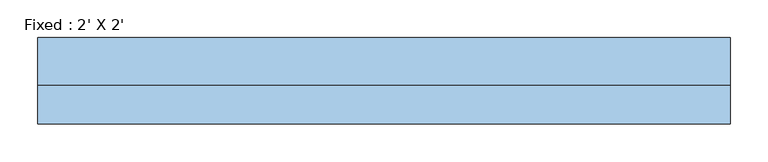
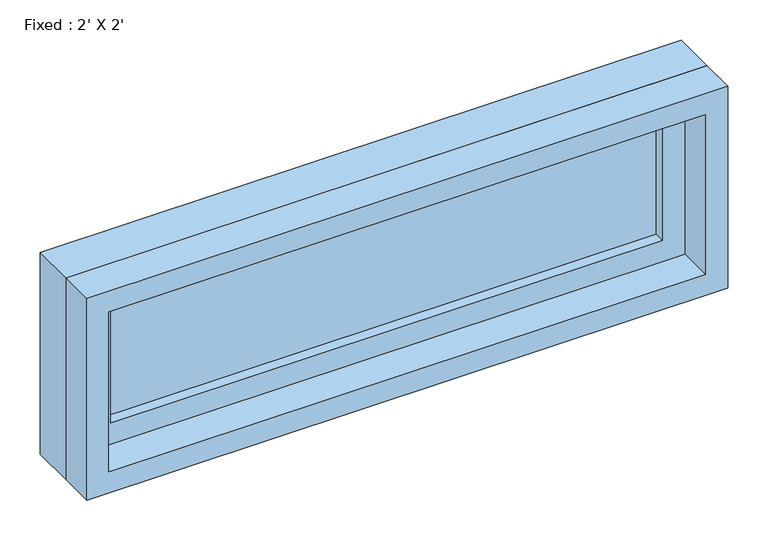
"""IFC4 building model written with IfcOpenShell, lengths in millimetres: window geometry, Fixed : 2' X 2'."""

from ifc_helpers import new_model, si_unit, frame, origin, place, context, project, spatial, polyline, outline, extrude, source, transform, mapped, element, save


def fixed_2_x_2_cd9169cd(model_context):
    return source(origin(), model_context, "Body", "SweptSolid", [
        extrude(outline(polyline([(355.6, 9.525), (-431.8, 9.525), (-431.8, 22.225), (355.6, 22.225), (355.6, 9.525)])), frame((0.0, 0.0, 368.3), z_axis=(0.0, 0.0, 1.0), x_axis=(1.0, 0.0, 0.0)), (0.0, 0.0, 1.0), 177.8),
        extrude(outline(polyline([(590.55, -476.25), (323.85, -476.25), (323.85, 400.05), (590.55, 400.05), (590.55, -476.25)]), holes=[polyline([(546.1, -431.8), (546.1, 355.6), (368.3, 355.6), (368.3, -431.8), (546.1, -431.8)])]), frame((0.0, -6.35, 0.0), z_axis=(0.0, 1.0, 0.0), x_axis=(0.0, 0.0, 1.0)), (0.0, 0.0, 1.0), 44.45),
        extrude(outline(polyline([(609.6, -495.3), (304.8, -495.3), (304.8, 419.1), (609.6, 419.1), (609.6, -495.3)]), holes=[polyline([(577.85, -463.55), (577.85, 387.35), (336.55, 387.35), (336.55, -463.55), (577.85, -463.55)])]), frame((0.0, -57.15, 0.0), z_axis=(0.0, 1.0, 0.0), x_axis=(0.0, 0.0, 1.0)), (0.0, 0.0, 1.0), 50.8),
        extrude(outline(polyline([(609.6, 419.1), (609.6, -495.3), (304.8, -495.3), (304.8, 419.1), (609.6, 419.1)]), holes=[polyline([(590.55, 400.05), (323.85, 400.05), (323.85, -476.25), (590.55, -476.25), (590.55, 400.05)])]), frame((0.0, -6.35, 0.0), z_axis=(0.0, 1.0, 0.0), x_axis=(0.0, 0.0, 1.0)), (0.0, 0.0, 1.0), 63.5),
    ])


if __name__ == "__main__":
    model = new_model("IFC4")
    model_context = context("Model", 3, world=origin())
    ifc_project = project(units=[si_unit("LENGTHUNIT", "METRE", prefix="MILLI")], contexts=[model_context])
    site = spatial("IfcSite", under=ifc_project)
    building = spatial("IfcBuilding", under=site)
    placement = place(None, origin())
    fixed_2_x_2_shape = fixed_2_x_2_cd9169cd(model_context)
    element("IfcWindow", 1, ObjectType="Fixed : 2' X 2'", at=placement, inside=building, context=model_context, shape_type="MappedRepresentation", body=[
        mapped(fixed_2_x_2_shape, transform((0.0, 0.0, 0.0), x_axis=(1.0, 0.0, 0.0), y_axis=(0.0, 1.0, 0.0), z_axis=(0.0, 0.0, 1.0))),
    ])
    save(model, "model.ifc")

# Revit data of these elements
# Type "Fixed : 2' X 2'"
#   Type Mark = "18"
#   Construction Type Id = "GSP4R"
#   Assembly Code = "B2020100"
#   Analytic Construction = "1/8 in Pilkington single glazing"
#   Visual Light Transmittance = 0.9
#   Solar Heat Gain Coefficient = 0.78
#   Heat Transfer Coefficient (U) = 0.6496 BTU/(h·ft²·°F)
#   Height = 1' - 0"
#   Default Sill Height = 1' - 0"
#   Width = 3' - 0"
#   Window Inset = 0' - 0 3/4"
#   Define Thermal Properties by = 1
#   Glass Pane Material = Glass
#   Sash Material = Sash
#   Wall Closure = (empty or 0)
# Element 1 (IfcWindow, "Fixed : 2' X 2'")
#   Materials on its faces: "Sash", "Glass"
# Materials
#   "Glass": class "Glass", colour RGB 0 128 192, transparency 0.75, Description = "Soda Lime Glass", Cost = 0
#   "Sash": class "Wood", colour RGB 224 178 126, transparency 0, Cost = 0
